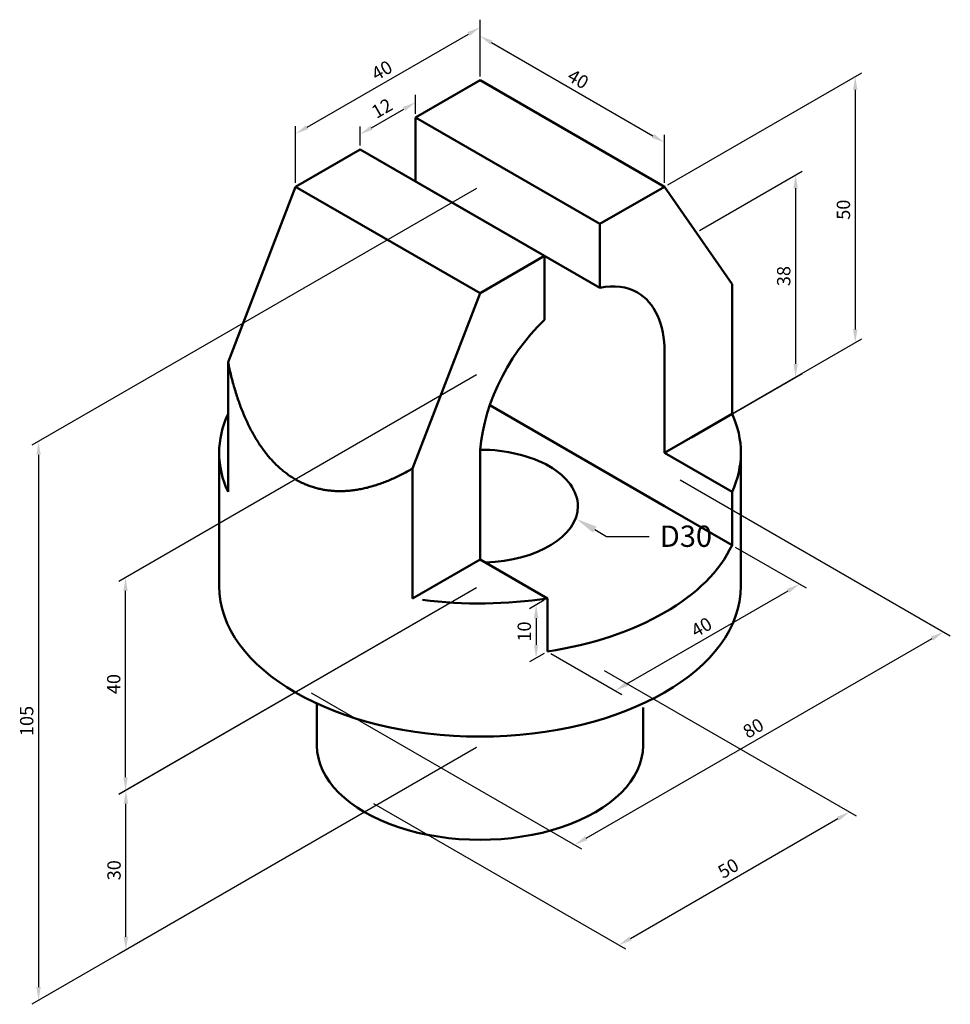
# Model space of a CAD drawing. Units: millimetres. Extents: x 2913 to 3088, y 3357 to 3542.
import ezdxf
from ezdxf import colors
from ezdxf.entities.mleader import LeaderData, LeaderLine
from ezdxf.math import Vec2, Vec3

# ---------------------------------------------------------------- set-up
doc = ezdxf.new("R2010")
doc.units = ezdxf.units.MM
for name, color, linetype, lineweight in [('M-DIMS', 2, 'Continuous', 25), ('M-OUTL', 7, 'Continuous', 50), ('M-TEXT', 3, 'Continuous', 25)]:
    doc.layers.add(name, color=color, linetype=linetype, lineweight=lineweight)
doc.styles.get("Standard").update_dxf_attribs({"font": 'arial.ttf'})
doc.dimstyles.new('ISO-25', dxfattribs={"dimtxt": 2.5, "dimasz": 2.5, "dimexe": 1.25, "dimexo": 0.625, "dimtad": 1, "dimtxsty": 'Standard', "dimcen": 2.5, "dimadec": 0, "dimazin": 0, "dimtfac": 1, "dimtmove": 0, "dimatfit": 3, "dimfxl": 1, "dimarcsym": 0})

# ---------------------------------------------------------------- blocks, each defined once
blk = doc.blocks.new('*D1')
at = {"layer": 'Defpoints', "color": 0, "transparency": 16777216}
for p in [(2987.52, 3526.28), (2987.52, 3523.44), (2977.13, 3517.44)]:
    blk.add_point(p, dxfattribs=at)
at = {"layer": 'M-DIMS', "color": 0, "lineweight": -2, "transparency": 16777216}
for p, q in [((2987.52, 3524.16), (2987.52, 3527.72)), ((2979.3, 3521.53), (2985.36, 3525.03)), ((2977.13, 3518.16), (2977.13, 3521.72))]:
    blk.add_line(p, q, dxfattribs=at)
at = {"layer": 'M-DIMS', "color": 0, "transparency": 16777216}
for points in [[(2985.15, 3525.39), (2985.57, 3524.67), (2987.52, 3526.28)], [(2979.09, 3521.89), (2979.51, 3521.17), (2977.13, 3520.28)]]:
    blk.add_solid(points, dxfattribs=at)
at = {"layer": 'M-DIMS', "color": 0, "transparency": 16777216, "insert": (2981.39, 3524.9), "char_height": 2.5, "attachment_point": 5, "rotation": 30}
blk.add_mtext('12', dxfattribs=at)
blk = doc.blocks.new('*D2')
at = {"layer": 'Defpoints', "color": 0, "transparency": 16777216}
for p in [(2999.65, 3540.37), (2999.65, 3530.44), (2965.01, 3510.44)]:
    blk.add_point(p, dxfattribs=at)
at = {"layer": 'M-DIMS', "color": 0, "lineweight": -2, "transparency": 16777216}
for p, q in [((2999.65, 3531.16), (2999.65, 3541.81)), ((2967.17, 3521.62), (2997.48, 3539.12)), ((2965.01, 3511.16), (2965.01, 3521.81))]:
    blk.add_line(p, q, dxfattribs=at)
at = {"layer": 'M-DIMS', "color": 0, "transparency": 16777216}
for points in [[(2997.28, 3539.48), (2997.69, 3538.76), (2999.65, 3540.37)], [(2966.96, 3521.98), (2967.38, 3521.26), (2965.01, 3520.37)]]:
    blk.add_solid(points, dxfattribs=at)
at = {"layer": 'M-DIMS', "color": 0, "transparency": 16777216, "insert": (2981.38, 3532.02), "char_height": 2.5, "attachment_point": 5, "rotation": 30}
blk.add_mtext('40', dxfattribs=at)
blk = doc.blocks.new('*D3')
at = {"layer": 'Defpoints', "color": 0, "transparency": 16777216}
for p in [(2999.65, 3530.44), (3034.29, 3518.75), (3034.29, 3510.44)]:
    blk.add_point(p, dxfattribs=at)
at = {"layer": 'M-DIMS', "color": 0, "lineweight": -2, "transparency": 16777216}
for p, q in [((2999.65, 3531.16), (2999.65, 3540.19)), ((3001.81, 3537.5), (3032.12, 3520)), ((3034.29, 3511.16), (3034.29, 3520.19))]:
    blk.add_line(p, q, dxfattribs=at)
at = {"layer": 'M-DIMS', "color": 0, "transparency": 16777216}
for points in [[(3002.02, 3537.86), (3001.61, 3537.13), (2999.65, 3538.75)], [(3032.33, 3520.36), (3031.92, 3519.63), (3034.29, 3518.75)]]:
    blk.add_solid(points, dxfattribs=at)
at = {"layer": 'M-DIMS', "color": 0, "transparency": 16777216, "insert": (3017.92, 3530.39), "char_height": 2.5, "attachment_point": 5, "rotation": 330}
blk.add_mtext('40', dxfattribs=at)
blk = doc.blocks.new('*D4')
at = {"layer": 'Defpoints', "color": 0, "transparency": 16777216}
for p in [(3040.23, 3501.87), (3058.91, 3474.65), (3040.23, 3463.87)]:
    blk.add_point(p, dxfattribs=at)
at = {"layer": 'M-DIMS', "color": 0, "lineweight": -2, "transparency": 16777216}
for p, q in [((3040.85, 3502.23), (3060.16, 3513.37)), ((3058.91, 3510.15), (3058.91, 3477.15)), ((3040.85, 3464.23), (3060.16, 3475.37))]:
    blk.add_line(p, q, dxfattribs=at)
at = {"layer": 'M-DIMS', "color": 0, "transparency": 16777216}
for points in [[(3058.49, 3510.15), (3059.32, 3510.15), (3058.91, 3512.65)], [(3058.49, 3477.15), (3059.32, 3477.15), (3058.91, 3474.65)]]:
    blk.add_solid(points, dxfattribs=at)
at = {"layer": 'M-DIMS', "color": 0, "transparency": 16777216, "insert": (3057, 3493.65), "char_height": 2.5, "attachment_point": 5, "rotation": 90}
blk.add_mtext('38', dxfattribs=at)
blk = doc.blocks.new('*D5')
at = {"layer": 'Defpoints', "color": 0, "transparency": 16777216}
for p in [(3034.29, 3510.44), (3070.11, 3481.12), (3034.29, 3460.44)]:
    blk.add_point(p, dxfattribs=at)
at = {"layer": 'M-DIMS', "color": 0, "lineweight": -2, "transparency": 16777216}
for p, q in [((3034.91, 3510.8), (3071.36, 3531.84)), ((3070.11, 3528.62), (3070.11, 3483.62)), ((3034.91, 3460.8), (3071.36, 3481.84))]:
    blk.add_line(p, q, dxfattribs=at)
at = {"layer": 'M-DIMS', "color": 0, "transparency": 16777216}
for points in [[(3069.69, 3528.62), (3070.53, 3528.62), (3070.11, 3531.12)], [(3069.69, 3483.62), (3070.53, 3483.62), (3070.11, 3481.12)]]:
    blk.add_solid(points, dxfattribs=at)
at = {"layer": 'M-DIMS', "color": 0, "transparency": 16777216, "insert": (3068.21, 3506.12), "char_height": 2.5, "attachment_point": 5, "rotation": 90}
blk.add_mtext('50', dxfattribs=at)
blk = doc.blocks.new('*D6')
at = {"layer": 'Defpoints', "color": 0, "transparency": 16777216}
for p in [(3046.97, 3443.12), (3059.67, 3435.78), (3012.33, 3423.12)]:
    blk.add_point(p, dxfattribs=at)
at = {"layer": 'M-DIMS', "color": 0, "lineweight": -2, "transparency": 16777216}
for p, q in [((3047.59, 3442.76), (3060.92, 3435.06)), ((3027.19, 3417.03), (3057.5, 3434.53)), ((3012.95, 3422.76), (3026.28, 3415.06))]:
    blk.add_line(p, q, dxfattribs=at)
at = {"layer": 'M-DIMS', "color": 0, "transparency": 16777216}
for points in [[(3057.3, 3434.9), (3057.71, 3434.17), (3059.67, 3435.78)], [(3026.99, 3417.4), (3027.4, 3416.67), (3025.03, 3415.78)]]:
    blk.add_solid(points, dxfattribs=at)
at = {"layer": 'M-DIMS', "color": 0, "transparency": 16777216, "insert": (3041.4, 3427.43), "char_height": 2.5, "attachment_point": 5, "rotation": 30}
blk.add_mtext('40', dxfattribs=at)
blk = doc.blocks.new('*D7')
at = {"layer": 'Defpoints', "color": 0, "transparency": 16777216}
for p in [(3012.33, 3433.12), (3010.19, 3421.88), (3012.33, 3423.12)]:
    blk.add_point(p, dxfattribs=at)
at = {"layer": 'M-DIMS', "color": 0, "lineweight": -2, "transparency": 16777216}
for p, q in [((3011.7, 3432.76), (3008.94, 3431.16)), ((3010.19, 3429.38), (3010.19, 3424.38)), ((3011.7, 3422.76), (3008.94, 3421.16))]:
    blk.add_line(p, q, dxfattribs=at)
at = {"layer": 'M-DIMS', "color": 0, "transparency": 16777216}
for points in [[(3009.77, 3429.38), (3010.61, 3429.38), (3010.19, 3431.88)], [(3009.77, 3424.38), (3010.61, 3424.38), (3010.19, 3421.88)]]:
    blk.add_solid(points, dxfattribs=at)
at = {"layer": 'M-DIMS', "color": 0, "transparency": 16777216, "insert": (3008.29, 3426.88), "char_height": 2.5, "attachment_point": 5, "rotation": 90}
blk.add_mtext('10', dxfattribs=at)
blk = doc.blocks.new('*D8')
at = {"layer": 'Defpoints', "color": 0, "transparency": 16777216}
for p in [(3036.63, 3455.73), (3086.71, 3426.81), (2967.34, 3415.73)]:
    blk.add_point(p, dxfattribs=at)
at = {"layer": 'M-DIMS', "color": 0, "lineweight": -2, "transparency": 16777216}
for p, q in [((3037.25, 3455.37), (3087.96, 3426.09)), ((3019.59, 3388.06), (3084.54, 3425.56)), ((2967.97, 3415.37), (3018.68, 3386.09))]:
    blk.add_line(p, q, dxfattribs=at)
at = {"layer": 'M-DIMS', "color": 0, "transparency": 16777216}
for points in [[(3084.33, 3425.92), (3084.75, 3425.2), (3086.71, 3426.81)], [(3019.38, 3388.42), (3019.8, 3387.7), (3017.43, 3386.81)]]:
    blk.add_solid(points, dxfattribs=at)
at = {"layer": 'M-DIMS', "color": 0, "transparency": 16777216, "insert": (3051.12, 3408.46), "char_height": 2.5, "attachment_point": 5, "rotation": 30}
blk.add_mtext('80', dxfattribs=at)
blk = doc.blocks.new('*D9')
at = {"layer": 'Defpoints', "color": 0, "transparency": 16777216}
for p in [(3022.31, 3419.95), (2979.01, 3394.95), (3069.03, 3392.98)]:
    blk.add_point(p, dxfattribs=at)
at = {"layer": 'M-DIMS', "color": 0, "lineweight": -2, "transparency": 16777216}
for p, q in [((3022.94, 3419.59), (3070.28, 3392.26)), ((2979.64, 3394.59), (3026.98, 3367.26)), ((3027.9, 3369.23), (3066.87, 3391.73))]:
    blk.add_line(p, q, dxfattribs=at)
at = {"layer": 'M-DIMS', "color": 0, "transparency": 16777216}
for points in [[(3066.66, 3392.09), (3067.08, 3391.37), (3069.03, 3392.98)], [(3027.69, 3369.59), (3028.11, 3368.87), (3025.73, 3367.98)]]:
    blk.add_solid(points, dxfattribs=at)
at = {"layer": 'M-DIMS', "color": 0, "transparency": 16777216, "insert": (3046.43, 3382.12), "char_height": 2.5, "attachment_point": 5, "rotation": 30}
blk.add_mtext('50', dxfattribs=at)
blk = doc.blocks.new('*D10')
at = {"layer": 'Defpoints', "color": 0, "transparency": 16777216}
for p in [(2999.65, 3435.44), (2999.65, 3405.44), (2933.15, 3397.04)]:
    blk.add_point(p, dxfattribs=at)
at = {"layer": 'M-DIMS', "color": 0, "lineweight": -2, "transparency": 16777216}
for p, q in [((2999.02, 3435.08), (2931.9, 3396.32)), ((2999.02, 3405.08), (2931.9, 3366.32)), ((2933.15, 3369.54), (2933.15, 3394.54))]:
    blk.add_line(p, q, dxfattribs=at)
at = {"layer": 'M-DIMS', "color": 0, "transparency": 16777216}
for points in [[(2932.73, 3394.54), (2933.57, 3394.54), (2933.15, 3397.04)], [(2932.73, 3369.54), (2933.57, 3369.54), (2933.15, 3367.04)]]:
    blk.add_solid(points, dxfattribs=at)
at = {"layer": 'M-DIMS', "color": 0, "transparency": 16777216, "insert": (2931.25, 3382.04), "char_height": 2.5, "attachment_point": 5, "rotation": 90}
blk.add_mtext('30', dxfattribs=at)
blk = doc.blocks.new('*D11')
at = {"layer": 'Defpoints', "color": 0, "transparency": 16777216}
for p in [(2999.65, 3475.44), (2933.09, 3437.01), (2999.65, 3435.44)]:
    blk.add_point(p, dxfattribs=at)
at = {"layer": 'M-DIMS', "color": 0, "lineweight": -2, "transparency": 16777216}
for p, q in [((2999.02, 3475.08), (2931.84, 3436.29)), ((2999.02, 3435.08), (2931.84, 3396.29)), ((2933.09, 3399.51), (2933.09, 3434.51))]:
    blk.add_line(p, q, dxfattribs=at)
at = {"layer": 'M-DIMS', "color": 0, "transparency": 16777216}
for points in [[(2932.67, 3434.51), (2933.5, 3434.51), (2933.09, 3437.01)], [(2932.67, 3399.51), (2933.5, 3399.51), (2933.09, 3397.01)]]:
    blk.add_solid(points, dxfattribs=at)
at = {"layer": 'M-DIMS', "color": 0, "transparency": 16777216, "insert": (2931.19, 3417.01), "char_height": 2.5, "attachment_point": 5, "rotation": 90}
blk.add_mtext('40', dxfattribs=at)
blk = doc.blocks.new('*D12')
at = {"layer": 'Defpoints', "color": 0, "transparency": 16777216}
for p in [(2999.65, 3510.44), (2999.65, 3405.44), (2916.75, 3357.58)]:
    blk.add_point(p, dxfattribs=at)
at = {"layer": 'M-DIMS', "color": 0, "lineweight": -2, "transparency": 16777216}
for p, q in [((2999.02, 3510.08), (2915.5, 3461.86)), ((2916.75, 3460.08), (2916.75, 3360.08)), ((2999.02, 3405.08), (2915.5, 3356.86))]:
    blk.add_line(p, q, dxfattribs=at)
at = {"layer": 'M-DIMS', "color": 0, "transparency": 16777216}
for points in [[(2916.34, 3460.08), (2917.17, 3460.08), (2916.75, 3462.58)], [(2916.34, 3360.08), (2917.17, 3360.08), (2916.75, 3357.58)]]:
    blk.add_solid(points, dxfattribs=at)
at = {"layer": 'M-DIMS', "color": 0, "transparency": 16777216, "insert": (2914.85, 3410.08), "char_height": 2.5, "attachment_point": 5, "rotation": 90}
blk.add_mtext('105', dxfattribs=at)

msp = doc.modelspace()

# ---------------------------------------------------------------- linework, layer by layer
at = {"layer": 'M-OUTL'}
for p, q in [((2999.649, 3530.437), (2987.524, 3523.437)), ((3034.29, 3510.437), (2999.649, 3530.437)), ((3022.166, 3503.437), (2987.524, 3523.437)), ((2987.524, 3523.437), (2987.524, 3511.437)), ((2977.132, 3517.437), (2965.008, 3510.437)), ((2977.132, 3517.437), (3011.773, 3497.437)), ((3022.166, 3491.437), (2977.132, 3517.437)), ((2965.008, 3510.437), (2952.328, 3477.495)), ((2965.008, 3510.437), (2999.649, 3490.437)), ((3022.166, 3503.437), (3034.29, 3510.437)), ((3034.29, 3510.437), (3046.969, 3492.131)), ((3022.166, 3503.437), (3022.166, 3491.437)), ((2999.649, 3490.437), (3011.773, 3497.437)), ((3011.773, 3497.437), (3011.773, 3485.437)), ((3046.969, 3467.758), (3046.969, 3492.131)), ((2999.649, 3490.437), (2986.969, 3457.495)), ((3022.166, 3491.437), (3022.166, 3491.435)), ((3011.775, 3485.433), (3011.77, 3485.443)), ((3011.773, 3485.437), (3011.775, 3485.433)), ((3034.29, 3480.437), (3034.29, 3470.437)), ((3034.29, 3480.437), (3034.29, 3460.437)), ((2952.328, 3453.117), (2952.328, 3477.495)), ((3034.29, 3460.437), (3034.29, 3470.437)), ((3034.29, 3450.437), (3001.485, 3469.377)), ((3034.29, 3460.437), (3046.969, 3467.758)), ((3034.29, 3460.437), (3034.29, 3466.828)), ((3039.436, 3463.408), (3046.969, 3467.758)), ((3039.436, 3463.408), (3039.436, 3463.408)), ((2950.659, 3435.437), (2950.659, 3460.437)), ((2999.649, 3459.357), (2999.649, 3440.437)), ((3034.29, 3460.437), (3046.969, 3453.117)), ((3048.639, 3435.437), (3048.639, 3460.437)), ((2986.969, 3433.117), (2986.969, 3457.495)), ((3046.969, 3443.117), (3046.969, 3453.117)), ((3034.29, 3450.437), (3046.969, 3443.117)), ((2986.969, 3433.117), (2999.649, 3440.437)), ((2999.649, 3440.437), (3012.328, 3433.117)), ((3012.328, 3423.117), (3012.328, 3433.117)), ((2969.03, 3405.437), (2969.03, 3413.358)), ((3030.267, 3412.632), (3030.267, 3405.437))]:
    msp.add_line(p, q, dxfattribs=at)
for points in [[(2965.008, 3455.437), (2964.822, 3455.555), (2964.637, 3455.674), (2964.452, 3455.792), (2964.266, 3455.91), (2964.081, 3456.028), (2963.896, 3456.147), (2963.711, 3456.267), (2963.533, 3456.404), (2963.355, 3456.54), (2963.177, 3456.677), (2962.999, 3456.813), (2962.821, 3456.949), (2962.643, 3457.086), (2962.467, 3457.227), (2962.297, 3457.382), (2962.126, 3457.536), (2961.956, 3457.691), (2961.785, 3457.845), (2961.615, 3458), (2961.444, 3458.154), (2961.277, 3458.316), (2961.115, 3458.488), (2960.952, 3458.661), (2960.789, 3458.833), (2960.627, 3459.005), (2960.464, 3459.177), (2960.301, 3459.349), (2960.143, 3459.532), (2959.989, 3459.721), (2959.834, 3459.911), (2959.68, 3460.101), (2959.525, 3460.291), (2959.37, 3460.48), (2959.216, 3460.67), (2959.067, 3460.872), (2958.921, 3461.079), (2958.774, 3461.286), (2958.628, 3461.493), (2958.482, 3461.7), (2958.335, 3461.907), (2958.189, 3462.114), (2958.05, 3462.336), (2957.912, 3462.56), (2957.774, 3462.784), (2957.636, 3463.008), (2957.498, 3463.232), (2957.36, 3463.456), (2957.222, 3463.68), (2957.093, 3463.921), (2956.964, 3464.162), (2956.835, 3464.402), (2956.705, 3464.643), (2956.576, 3464.884), (2956.447, 3465.124), (2956.319, 3465.367), (2956.199, 3465.624), (2956.078, 3465.881), (2955.958, 3466.138), (2955.837, 3466.396), (2955.717, 3466.653), (2955.597, 3466.91), (2955.479, 3467.171), (2955.367, 3467.444), (2955.256, 3467.717), (2955.144, 3467.99), (2955.033, 3468.263), (2954.922, 3468.536), (2954.81, 3468.809), (2954.703, 3469.089), (2954.601, 3469.378), (2954.498, 3469.666), (2954.396, 3469.955), (2954.294, 3470.243), (2954.192, 3470.532), (2954.089, 3470.821), (2953.992, 3471.118), (2953.899, 3471.422), (2953.806, 3471.726), (2953.714, 3472.029), (2953.621, 3472.333), (2953.528, 3472.637), (2953.435, 3472.941), (2953.349, 3473.255), (2953.265, 3473.574), (2953.181, 3473.892), (2953.098, 3474.211), (2953.014, 3474.529), (2952.931, 3474.848), (2952.847, 3475.167), (2952.772, 3475.497), (2952.698, 3475.83), (2952.624, 3476.163), (2952.55, 3476.496), (2952.476, 3476.829), (2952.402, 3477.162), (2952.328, 3477.495)], [(2986.969, 3457.495), (2986.713, 3457.353), (2986.456, 3457.211), (2986.199, 3457.069), (2985.942, 3456.927), (2985.686, 3456.785), (2985.429, 3456.643), (2985.173, 3456.504), (2984.919, 3456.38), (2984.665, 3456.256), (2984.411, 3456.132), (2984.157, 3456.008), (2983.904, 3455.885), (2983.65, 3455.761), (2983.397, 3455.642), (2983.146, 3455.537), (2982.896, 3455.431), (2982.645, 3455.326), (2982.395, 3455.22), (2982.144, 3455.114), (2981.894, 3455.009), (2981.645, 3454.911), (2981.398, 3454.824), (2981.151, 3454.737), (2980.905, 3454.65), (2980.658, 3454.563), (2980.411, 3454.476), (2980.164, 3454.389), (2979.919, 3454.313), (2979.677, 3454.244), (2979.434, 3454.176), (2979.191, 3454.107), (2978.948, 3454.039), (2978.705, 3453.97), (2978.462, 3453.902), (2978.223, 3453.846), (2977.984, 3453.797), (2977.746, 3453.747), (2977.507, 3453.697), (2977.269, 3453.647), (2977.03, 3453.597), (2976.791, 3453.548), (2976.557, 3453.514), (2976.323, 3453.483), (2976.089, 3453.452), (2975.855, 3453.421), (2975.622, 3453.39), (2975.388, 3453.358), (2975.154, 3453.327), (2974.925, 3453.315), (2974.696, 3453.303), (2974.467, 3453.291), (2974.239, 3453.278), (2974.01, 3453.266), (2973.781, 3453.254), (2973.553, 3453.244), (2973.329, 3453.251), (2973.106, 3453.257), (2972.882, 3453.264), (2972.659, 3453.27), (2972.435, 3453.277), (2972.212, 3453.283), (2971.99, 3453.295), (2971.772, 3453.32), (2971.554, 3453.346), (2971.336, 3453.371), (2971.118, 3453.396), (2970.9, 3453.422), (2970.682, 3453.447), (2970.467, 3453.48), (2970.255, 3453.524), (2970.043, 3453.569), (2969.831, 3453.613), (2969.619, 3453.657), (2969.407, 3453.701), (2969.195, 3453.745), (2968.987, 3453.8), (2968.781, 3453.862), (2968.575, 3453.925), (2968.369, 3453.988), (2968.164, 3454.051), (2967.958, 3454.113), (2967.752, 3454.176), (2967.551, 3454.252), (2967.352, 3454.334), (2967.153, 3454.415), (2966.953, 3454.496), (2966.754, 3454.578), (2966.555, 3454.659), (2966.356, 3454.741), (2966.162, 3454.838), (2965.97, 3454.938), (2965.778, 3455.038), (2965.585, 3455.137), (2965.393, 3455.237), (2965.2, 3455.337), (2965.008, 3455.437)]]:
    msp.add_lwpolyline(points, dxfattribs=at)
for centre, major_axis, start_param, end_param in [((3016.969, 3469.358), (-12.247, -21.213), 3.1415927, 3.6222982), ((3016.969, 3469.358), (-12.247, -21.213), 2.3561945, 3.1415927), ((3016.969, 3469.358), (-12.247, -21.213), 4.2316835, 5.4977871), ((2999.649, 3460.437), (-48.99, 0), 6.0213859, 6.2831853), ((2999.649, 3460.437), (-48.99, 0), 9.1629786, 9.6865773), ((2999.649, 3450.437), (18.371, 0), 0.7853982, 1.5675773), ((2999.649, 3460.437), (-48.99, 0), 0, 0.2617994), ((2999.649, 3450.437), (18.371, 0), 0, 0.7853982), ((2999.649, 3450.437), (18.371, 0), 4.7680595, 6.2831853), ((2999.649, 3450.437), (-48.99, 0), 8.115781, 9.1629786), ((2999.649, 3435.437), (48.99, 0), 3.1415927, 6.2831853), ((2999.649, 3460.437), (-48.99, 0), 7.6315656, 8.115781), ((2999.649, 3405.437), (-30.619, 0), 0, 3.1415927)]:
    msp.add_ellipse(centre, major_axis=major_axis, ratio=0.5773503, start_param=start_param, end_param=end_param, dxfattribs=at)

# ---------------------------------------------------------------- dimensions: what is measured, and where the dimension line sits
at = {"layer": 'M-DIMS'}
for p1, p2, distance, picture, middle in [((2965.008, 3510.437), (2999.649, 3530.437), 8.603, '*D2', (2981.378, 3532.018)), ((2999.649, 3530.437), (3034.29, 3510.437), 7.196, '*D3', (3017.92, 3530.392)), ((3034.29, 3510.437), (3034.29, 3460.437), 35.822, '*D5', (3068.21, 3506.119)), ((2977.132, 3517.437), (2987.524, 3523.437), 2.458, '*D1', (2981.388, 3524.904)), ((3040.227, 3501.865), (3040.227, 3463.865), 18.678, '*D4', (3057.003, 3493.649)), ((2999.649, 3510.437), (2999.649, 3405.437), -82.894, '*D12', (2914.853, 3410.078)), ((2999.649, 3435.437), (2999.649, 3475.437), 66.562, '*D11', (2931.186, 3417.008)), ((2967.343, 3415.726), (3036.625, 3455.726), -50.083, '*D8', (3051.116, 3408.458)), ((3012.328, 3423.117), (3046.969, 3443.117), -12.7, '*D6', (3041.398, 3427.431)), ((2999.649, 3405.437), (2999.649, 3435.437), 66.499, '*D10', (2931.247, 3382.044)), ((3012.328, 3433.117), (3012.328, 3423.117), -2.139, '*D7', (3008.288, 3426.881)), ((2979.012, 3394.953), (3022.313, 3419.953), -46.722, '*D9', (3046.434, 3382.124))]:
    dim = msp.add_aligned_dim(p1=p1, p2=p2, distance=distance, dimstyle='ISO-25', override={"dimclrd": 0, "dimclre": 0, "dimclrt": 0}, dxfattribs=at)
    dim.commit()
    dim.dimension.update_dxf_attribs({"geometry": picture, "text_midpoint": middle})

# ---------------------------------------------------------------- leaders
at = {"layer": 'M-TEXT'}
ml = msp.add_multileader_mtext('Standard', dxfattribs=at)
ml.set_content('D30', color=256)
ml.set_leader_properties()
ml.build(insert=Vec2(0, 0))
ctx = ml.context
ctx.base_point, ctx.plane_origin = Vec3(3031.41, 3444.752), Vec3(3017.733, 3448.03)
notes = []
notes.append((ctx, [(0, (1, 1, 0), (3023.41, 3444.752), (1, 0), 8, [(0, [(3017.733, 3448.03)], 0, [])])]))
ctx.mtext.insert, ctx.mtext.flow_direction = Vec3(3033.41, 3446.787), 5
for ctx, leaders in notes:
    for number, flags, end, landing, length, lines in leaders:
        leader = LeaderData()
        leader.index, (leader.has_last_leader_line, leader.has_dogleg_vector, leader.attachment_direction) = number, flags
        leader.last_leader_point, leader.dogleg_vector, leader.dogleg_length = Vec3(end), Vec3(landing), length
        for number, points, colour, breaks in lines:
            line = LeaderLine()
            line.index, line.vertices, line.color, line.breaks = number, Vec3.list(points), colors.encode_raw_color(colour), breaks
            leader.lines.append(line)
        ctx.leaders.append(leader)

doc.saveas('drawing.dxf')
